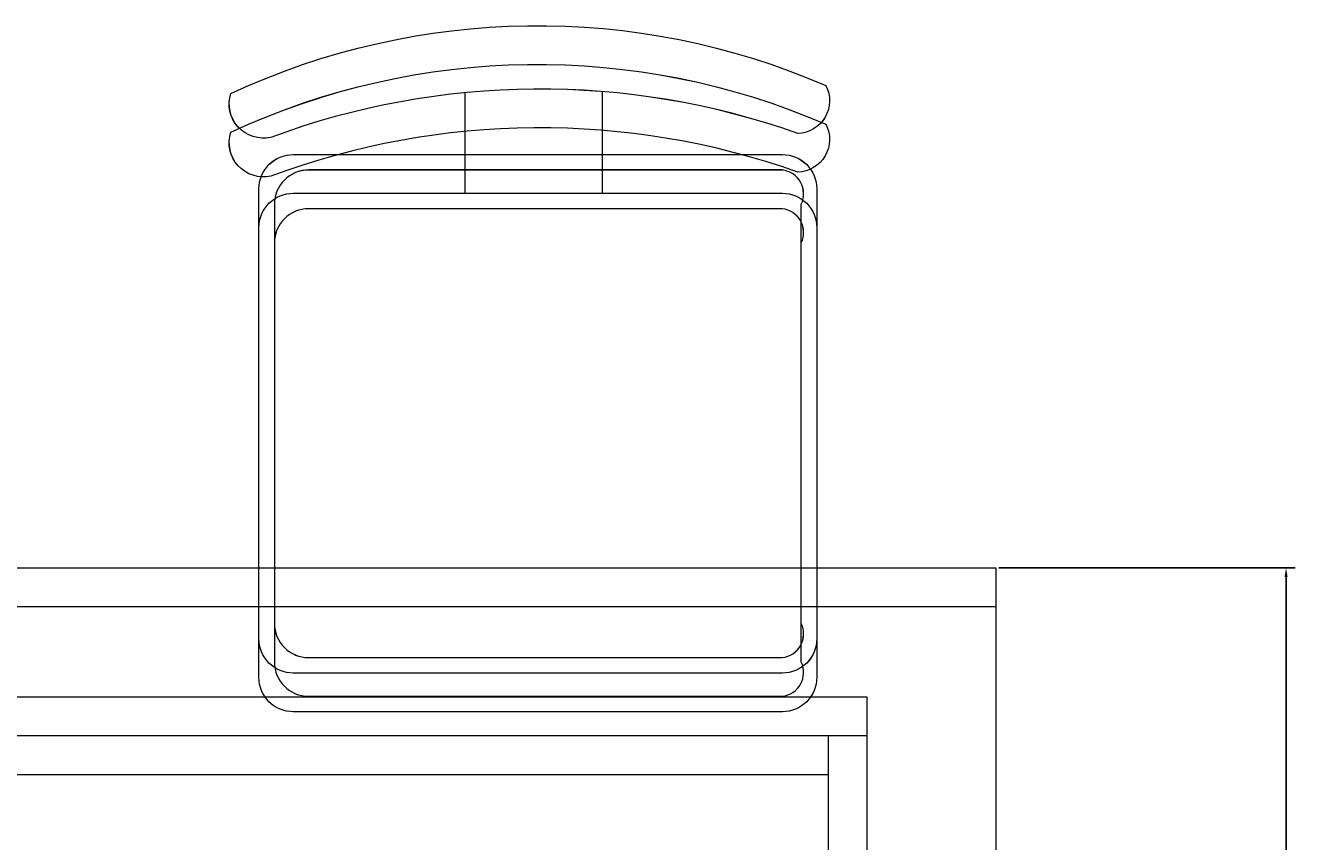
# Model space of a CAD drawing. Units: inches. Extents: x 1885 to 2748, y 783 to 2421.
# Tile 26 of 117: x 2367 to 2392, y 1274 to 1290. Entities that reach past the tile are written whole.
import ezdxf

# ---------------------------------------------------------------- set-up
doc = ezdxf.new("R2010")
doc.units = ezdxf.units.IN
doc.layers.add('A-ANNO-DIMS', color=2, linetype='Continuous', lineweight=18)
doc.layers.add('A-FURN', color=8, linetype='Continuous', lineweight=13)
doc.styles.get("Standard").update_dxf_attribs({"font": 'arial.ttf'})
doc.dimstyles.get("Standard").update_dxf_attribs({"dimtxt": 0.18, "dimasz": 0.18, "dimexe": 0.18, "dimexo": 0.0625, "dimgap": 0.09, "dimtad": 0, "dimtih": 1, "dimtoh": 1, "dimdec": 4, "dimzin": 0, "dimdsep": 46, "dimtxsty": 'Standard', "dimcen": 0.09, "dimadec": 0, "dimazin": 0, "dimtfac": 1, "dimtdec": 4, "dimtofl": 0, "dimtmove": 0, "dimatfit": 3, "dimfxl": 1, "dimtolj": 1, "dimtzin": 0, "dimarcsym": 0})

# ---------------------------------------------------------------- blocks, each defined once
blk = doc.blocks.new('TABLE-DINING-RECT')
for points in [[(-0.004, 23.421), (37.776, 23.421), (37.776, 0.754), (-0.004, 0.754)], [(-0.004, 23.421), (37.776, 23.421), (37.776, 0.753), (-0.004, 0.753)], [(-0.004, 22.666), (37.776, 22.666), (37.776, -0.002), (-0.004, -0.002)], [(-0.004, 22.665), (37.776, 22.665), (37.776, -0.002), (-0.004, -0.002)], [(2.515, 20.903), (35.257, 20.903), (35.257, 3.272), (2.515, 3.272)], [(2.515, 20.902), (35.257, 20.902), (35.257, 3.272), (2.515, 3.272)], [(2.515, 20.147), (35.257, 20.147), (35.257, 2.517), (2.515, 2.517)], [(2.515, 20.147), (35.257, 20.147), (35.257, 2.516), (2.515, 2.516)], [(3.27, 20.147), (34.501, 20.147), (34.501, 4.028), (3.27, 4.028)], [(3.27, 20.147), (34.501, 20.147), (34.501, 4.027), (3.27, 4.027)], [(3.27, 19.391), (34.501, 19.391), (34.501, 3.272), (3.27, 3.272)], [(3.27, 19.391), (34.501, 19.391), (34.501, 3.272), (3.27, 3.272)]]:
    blk.add_lwpolyline(points, close=True)
blk = doc.blocks.new('*D36')
at = {"layer": 'A-ANNO-DIMS', "color": 0, "lineweight": -2, "transparency": 16777216}
for p, q in [((2386.478, 1279.691), (2392.263, 1279.691)), ((2392.083, 1279.511), (2392.083, 1268.161)), ((2392.083, 1256.448), (2392.083, 1267.797)), ((2386.478, 1256.268), (2392.263, 1256.268))]:
    blk.add_line(p, q, dxfattribs=at)
at = {"layer": 'A-ANNO-DIMS', "color": 0, "transparency": 16777216}
for points in [[(2392.053, 1279.511), (2392.113, 1279.511), (2392.083, 1279.691)], [(2392.053, 1256.448), (2392.113, 1256.448), (2392.083, 1256.268)]]:
    blk.add_solid(points, dxfattribs=at)
at = {"layer": 'Defpoints', "color": 0, "transparency": 16777216}
for p in [(2386.416, 1279.691), (2392.083, 1279.691), (2386.416, 1256.268)]:
    blk.add_point(p, dxfattribs=at)
at = {"layer": 'A-ANNO-DIMS', "color": 0, "transparency": 16777216, "insert": (2392.083, 1267.979), "char_height": 0.18, "attachment_point": 5}
blk.add_mtext('\\A1;23 TYP.', dxfattribs=at)

msp = doc.modelspace()

# ---------------------------------------------------------------- linework, layer by layer
at = {"layer": 'A-FURN'}
for points in [[(2372.262, 1288.094, -0.578392), (2371.482, 1288.951, -0.214524), (2383.098, 1289.107, -0.552014), (2382.552, 1288.172, 0.175809), (2372.262, 1288.094)], [(2372.262, 1288.094, -0.578392), (2371.483, 1288.951, -0.214524), (2383.098, 1289.107, -0.552014), (2382.552, 1288.171, 0.175809), (2372.262, 1288.094)], [(2372.262, 1287.338, -0.578392), (2371.482, 1288.196, -0.214524), (2383.098, 1288.351, -0.552014), (2382.552, 1287.416, 0.175809), (2372.262, 1287.338)], [(2372.262, 1287.338, -0.578392), (2371.483, 1288.195, -0.214524), (2383.098, 1288.351, -0.552014), (2382.552, 1287.416, 0.175809), (2372.262, 1287.338)], [(2376.054, 1287.759), (2376.054, 1288.967, 0.064759)], [(2376.054, 1287.758), (2376.054, 1288.967, 0.064759)], [(2376.054, 1287.003), (2376.054, 1288.211, 0.064759)], [(2376.054, 1287.003), (2376.054, 1288.211, 0.064759)], [(2382.252, 1287.759, -0.414214), (2382.92, 1287.091), (2382.92, 1278.307, -0.414214), (2382.252, 1277.638), (2372.699, 1277.638, -0.414214), (2372.03, 1278.307), (2372.03, 1287.091, -0.414214), (2372.699, 1287.759), (2382.252, 1287.759)], [(2382.252, 1287.758, -0.414214), (2382.92, 1287.09), (2382.92, 1278.306, -0.414214), (2382.252, 1277.638), (2372.699, 1277.638, -0.414214), (2372.03, 1278.306), (2372.03, 1287.09, -0.414214), (2372.699, 1287.758), (2382.252, 1287.758)], [(2382.252, 1287.003, -0.414214), (2382.92, 1286.335), (2382.92, 1277.551, -0.414214), (2382.252, 1276.883), (2372.699, 1276.883, -0.414214), (2372.03, 1277.551), (2372.03, 1286.335, -0.414214), (2372.699, 1287.003), (2382.252, 1287.003)], [(2382.252, 1287.003, -0.414214), (2382.92, 1286.335), (2382.92, 1277.551, -0.414214), (2382.252, 1276.883), (2372.699, 1276.883, -0.414214), (2372.03, 1277.551), (2372.03, 1286.335, -0.414214), (2372.699, 1287.003), (2382.252, 1287.003)]]:
    msp.add_lwpolyline(points, format="xyb", dxfattribs=at)
for points in [[(2378.728, 1288.989), (2378.728, 1287.759)], [(2378.728, 1288.989), (2378.728, 1287.758)], [(2378.728, 1288.233), (2378.728, 1287.003)], [(2378.728, 1288.233), (2378.728, 1287.003)]]:
    msp.add_lwpolyline(points, dxfattribs=at)
for points in [[(2382.247, 1287.458), (2373, 1287.458, 0.414214), (2372.331, 1286.789), (2372.331, 1278.608, 0.414214), (2373, 1277.94), (2382.247, 1277.94, 0.512069), (2382.619, 1278.608), (2382.619, 1286.789, 0.512069)], [(2382.247, 1287.457), (2373, 1287.457, 0.414214), (2372.331, 1286.789), (2372.331, 1278.608, 0.414214), (2373, 1277.939), (2382.247, 1277.939, 0.512069), (2382.619, 1278.608), (2382.619, 1286.789, 0.512069)], [(2382.247, 1286.702), (2373, 1286.702, 0.414214), (2372.331, 1286.034), (2372.331, 1277.852, 0.414214), (2373, 1277.184), (2382.247, 1277.184, 0.512069), (2382.619, 1277.852), (2382.619, 1286.034, 0.512069)], [(2382.247, 1286.702), (2373, 1286.702, 0.414214), (2372.331, 1286.033), (2372.331, 1277.852, 0.414214), (2373, 1277.184), (2382.247, 1277.184, 0.512069), (2382.619, 1277.852), (2382.619, 1286.033, 0.512069)]]:
    msp.add_lwpolyline(points, format="xyb", close=True, dxfattribs=at)

# ---------------------------------------------------------------- block references
msp.add_blockref('TABLE-DINING-RECT', (2348.64, 1256.27), dxfattribs=at)

# ---------------------------------------------------------------- dimensions: what is measured, and where the dimension line sits
at = {"layer": 'A-ANNO-DIMS'}
dim = msp.add_linear_dim(base=(2392.083, 1279.691), p1=(2386.416, 1256.268), p2=(2386.416, 1279.691), angle=90, text='<> TYP.', dimstyle='Standard', override={"dimdec": 0, "dimlfac": 1, "dimrnd": 0, "dimzin": 0, "dimdsep": 46, "dimlunit": 2}, dxfattribs=at)
dim.commit()
dim.dimension.update_dxf_attribs({"geometry": '*D36', "text_midpoint": (2392.083, 1267.979)})

doc.saveas('drawing.dxf')
